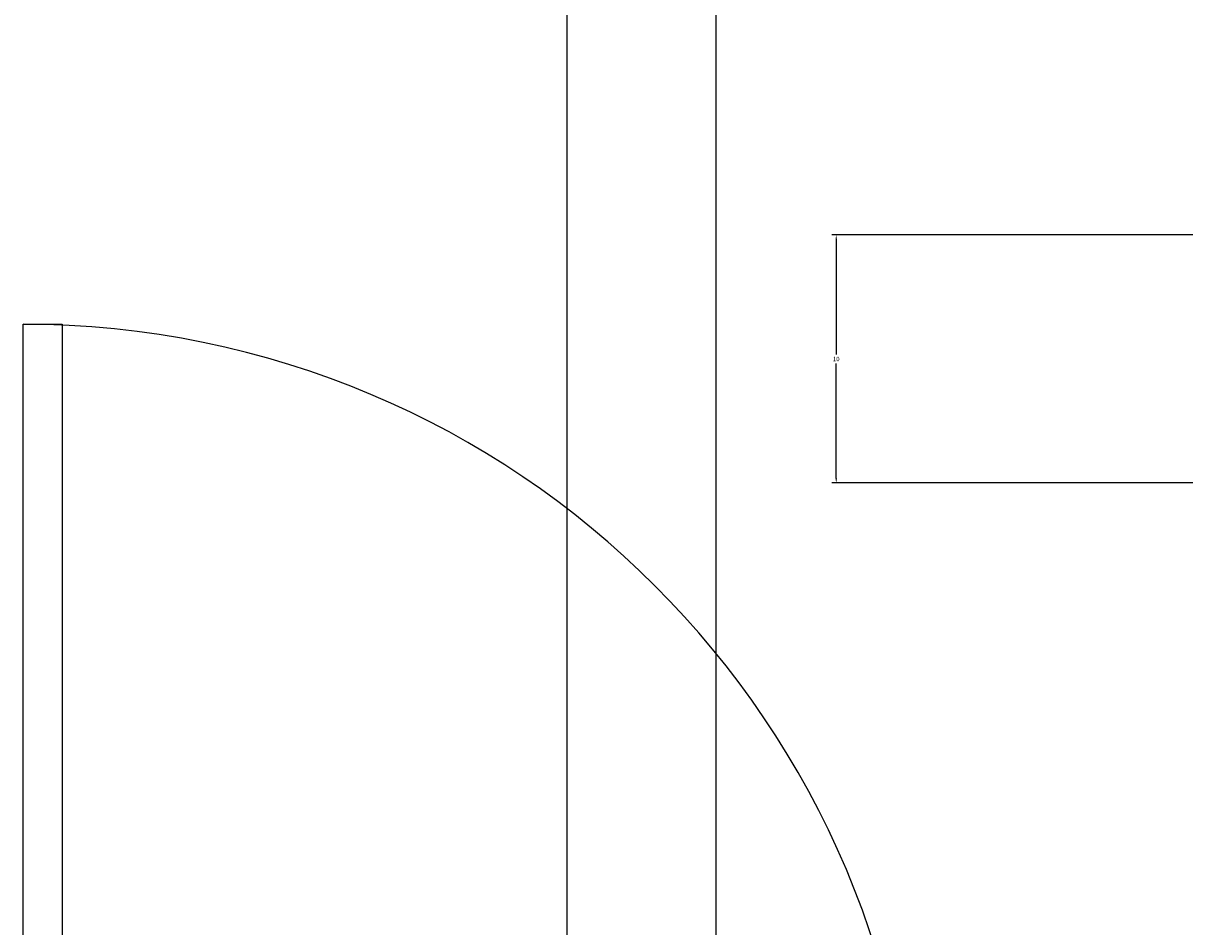
# Model space of a CAD drawing. Units: inches. Extents: x 2307 to 2544, y 2171 to 2540.
# Tile 9 of 52: x 2434 to 2481, y 2208 to 2244. Entities that reach past the tile are written whole.
import ezdxf

# ---------------------------------------------------------------- set-up
doc = ezdxf.new("R2010")
doc.units = ezdxf.units.IN
doc.layers.add('A-ANNO-DIMS', color=2, linetype='Continuous', lineweight=18)
doc.layers.add('A-DOOR', color=3, linetype='Continuous', lineweight=25)
doc.styles.get("Standard").update_dxf_attribs({"font": 'arial.ttf'})
doc.dimstyles.get("Standard").update_dxf_attribs({"dimtxt": 0.18, "dimasz": 0.18, "dimexe": 0.18, "dimexo": 0.0625, "dimgap": 0.09, "dimtad": 0, "dimtih": 1, "dimtoh": 1, "dimdec": 4, "dimzin": 0, "dimdsep": 46, "dimtxsty": 'Standard', "dimcen": 0.09, "dimadec": 0, "dimazin": 0, "dimtfac": 1, "dimtdec": 4, "dimtofl": 0, "dimtmove": 0, "dimatfit": 3, "dimfxl": 1, "dimtolj": 1, "dimtzin": 0, "dimarcsym": 0})

# ---------------------------------------------------------------- blocks, each defined once
blk = doc.blocks.new('*U13')
for p, q in [((0, 0), (0, -6)), ((40, 0), (40, -6))]:
    blk.add_line(p, q)
blk.add_lwpolyline([(0, 0), (0, 40), (1.75, 40), (1.75, 0)], close=True)
blk.add_arc((0, 0), 40, 0, 90)
blk = doc.blocks.new('*D53')
at = {"layer": 'A-ANNO-DIMS', "color": 0, "lineweight": -2, "transparency": 16777216}
for p, q in [((2455.696, 2439.447), (2455.696, 2171.18)), ((2461.696, 2439.447), (2461.696, 2171.18)), ((2455.876, 2171.36), (2458.546, 2171.36)), ((2461.516, 2171.36), (2458.845, 2171.36))]:
    blk.add_line(p, q, dxfattribs=at)
at = {"layer": 'A-ANNO-DIMS', "color": 0, "transparency": 16777216}
for points in [[(2455.876, 2171.39), (2455.876, 2171.33), (2455.696, 2171.36)], [(2461.516, 2171.39), (2461.516, 2171.33), (2461.696, 2171.36)]]:
    blk.add_solid(points, dxfattribs=at)
at = {"layer": 'Defpoints', "color": 0, "transparency": 16777216}
for p in [(2455.696, 2439.51), (2461.696, 2439.51), (2461.696, 2171.36)]:
    blk.add_point(p, dxfattribs=at)
at = {"layer": 'A-ANNO-DIMS', "color": 0, "transparency": 16777216, "insert": (2458.696, 2171.36), "char_height": 0.18, "attachment_point": 5}
blk.add_mtext('\\A1;6', dxfattribs=at)
blk = doc.blocks.new('*D54')
at = {"layer": 'A-ANNO-DIMS', "color": 0, "lineweight": -2, "transparency": 16777216}
for p, q in [((2461.696, 2435.447), (2461.696, 2171.18)), ((2491.696, 2435.447), (2491.696, 2171.18)), ((2461.876, 2171.36), (2476.477, 2171.36)), ((2491.516, 2171.36), (2476.914, 2171.36))]:
    blk.add_line(p, q, dxfattribs=at)
at = {"layer": 'A-ANNO-DIMS', "color": 0, "transparency": 16777216}
for points in [[(2461.876, 2171.39), (2461.876, 2171.33), (2461.696, 2171.36)], [(2491.516, 2171.39), (2491.516, 2171.33), (2491.696, 2171.36)]]:
    blk.add_solid(points, dxfattribs=at)
at = {"layer": 'Defpoints', "color": 0, "transparency": 16777216}
for p in [(2461.696, 2435.51), (2491.696, 2435.51), (2491.696, 2171.36)]:
    blk.add_point(p, dxfattribs=at)
at = {"layer": 'A-ANNO-DIMS', "color": 0, "transparency": 16777216, "insert": (2476.696, 2171.36), "char_height": 0.18, "attachment_point": 5}
blk.add_mtext('\\A1;30', dxfattribs=at)
blk = doc.blocks.new('*D58')
at = {"layer": 'A-ANNO-DIMS', "color": 0, "lineweight": -2, "transparency": 16777216}
for p, q in [((2485.633, 2235.51), (2466.366, 2235.51)), ((2466.546, 2235.33), (2466.546, 2230.691)), ((2466.546, 2225.69), (2466.546, 2230.328)), ((2485.633, 2225.51), (2466.366, 2225.51))]:
    blk.add_line(p, q, dxfattribs=at)
at = {"layer": 'A-ANNO-DIMS', "color": 0, "transparency": 16777216}
for points in [[(2466.516, 2235.33), (2466.576, 2235.33), (2466.546, 2235.51)], [(2466.516, 2225.69), (2466.576, 2225.69), (2466.546, 2225.51)]]:
    blk.add_solid(points, dxfattribs=at)
at = {"layer": 'Defpoints', "color": 0, "transparency": 16777216}
for p in [(2466.546, 2235.51), (2485.696, 2235.51), (2485.696, 2225.51)]:
    blk.add_point(p, dxfattribs=at)
at = {"layer": 'A-ANNO-DIMS', "color": 0, "transparency": 16777216, "insert": (2466.546, 2230.51), "char_height": 0.18, "attachment_point": 5}
blk.add_mtext('\\A1;10', dxfattribs=at)

msp = doc.modelspace()

# ---------------------------------------------------------------- block references
at = {"layer": 'A-DOOR', "xscale": 0.9, "yscale": 0.9, "zscale": 0.9}
msp.add_blockref('*U13', (2433.7832, 2195.9096), dxfattribs=at)

# ---------------------------------------------------------------- dimensions: what is measured, and where the dimension line sits
at = {"layer": 'A-ANNO-DIMS'}
for base, p1, p2, picture, middle in [((2461.6958, 2171.3596), (2455.6958, 2439.5096), (2461.6958, 2439.5096), '*D53', (2458.6958, 2171.3596)), ((2491.6958, 2171.3596), (2461.6958, 2435.5096), (2491.6958, 2435.5096), '*D54', (2476.6958, 2171.3596))]:
    dim = msp.add_linear_dim(base=base, p1=p1, p2=p2, dimstyle='Standard', override={"dimdec": 0, "dimlfac": 1, "dimrnd": 0, "dimzin": 0, "dimdsep": 46, "dimlunit": 2}, dxfattribs=at)
    dim.commit()
    dim.dimension.update_dxf_attribs({"geometry": picture, "text_midpoint": middle})
dim = msp.add_linear_dim(base=(2466.5458, 2235.5096), p1=(2485.6958, 2225.5096), p2=(2485.6958, 2235.5096), angle=90, dimstyle='Standard', override={"dimdec": 0, "dimlfac": 1, "dimrnd": 0, "dimzin": 0, "dimdsep": 46, "dimlunit": 2}, dxfattribs=at)
dim.commit()
dim.dimension.update_dxf_attribs({"geometry": '*D58', "text_midpoint": (2466.5458, 2230.5096)})

doc.saveas('drawing.dxf')
